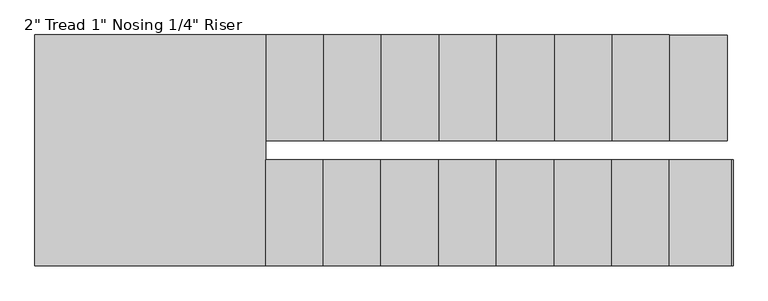
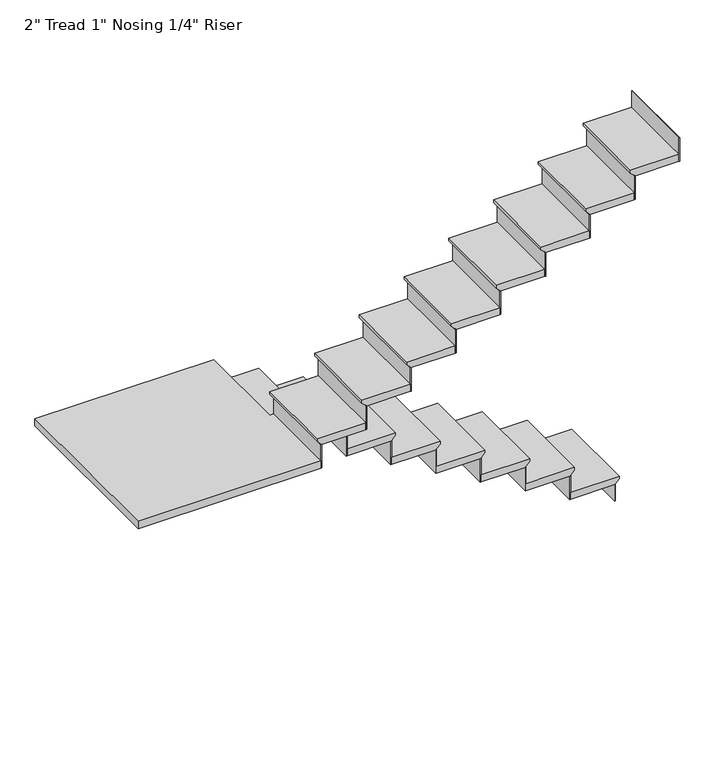
"""IFC4 building model written with IfcOpenShell, lengths in millimetres: stair flight geometry."""

from ifc_helpers import new_model, si_unit, origin, place, context, project, spatial, faceted_brep, source, transform, mapped, element, save


def stair_flight_bb5844b6(model_context):
    return source(origin(), model_context, "Body", "Brep", [
        faceted_brep([(-1805.9198569, -5306.3933037, 150.2833333), (-1805.9198569, -5306.3933037, 169.3333333), (-1805.9198569, -5865.1933037, 169.3333333), (-1805.9198569, -5865.1933037, 150.2833333), (-1831.3198569, -5306.3933037, 124.8833333), (-1831.3198569, -5865.1933037, 124.8833333), (-2136.1198569, -5306.3933037, 169.3333333), (-2136.1198569, -5865.1933037, 169.3333333), (-1831.3198569, -5865.1933037, 118.5333333), (-2136.1198569, -5865.1933037, 118.5333333), (-2136.1198569, -5306.3933037, 118.5333333), (-1831.3198569, -5306.3933037, 118.5333333)], [[[0, 1, 2, 3]], [[4, 0, 3, 5]], [[2, 1, 6, 7]], [[8, 9, 10, 11]], [[2, 7, 9, 8, 5, 3]], [[8, 11, 4, 5]], [[6, 1, 0, 4, 11, 10]], [[7, 6, 10, 9]]]),
        faceted_brep([(-1831.3198569, -5306.3933037, 118.5333333), (-1831.3198569, -5306.3933037, 0.0), (-1837.6698569, -5306.3933037, 0.0), (-1837.6698569, -5306.3933037, 118.5333333), (-1831.3198569, -5865.1933037, 118.5333333), (-1837.6698569, -5865.1933037, 118.5333333), (-1837.6698569, -5865.1933037, 0.0), (-1831.3198569, -5865.1933037, 0.0)], [[[0, 1, 2, 3]], [[4, 5, 6, 7]], [[1, 0, 4, 7]], [[2, 1, 7, 6]], [[3, 2, 6, 5]], [[0, 3, 5, 4]]]),
        faceted_brep([(-2136.1198569, -5306.3933037, 287.8666667), (-2136.1198569, -5306.3933037, 118.5333333), (-2142.4698569, -5306.3933037, 118.5333333), (-2142.4698569, -5306.3933037, 287.8666667), (-2136.1198569, -5865.1933037, 287.8666667), (-2142.4698569, -5865.1933037, 287.8666667), (-2142.4698569, -5865.1933037, 118.5333333), (-2136.1198569, -5865.1933037, 118.5333333)], [[[0, 1, 2, 3]], [[4, 5, 6, 7]], [[1, 0, 4, 7]], [[2, 1, 7, 6]], [[3, 2, 6, 5]], [[0, 3, 5, 4]]]),
        faceted_brep([(-2110.7198569, -5865.1933037, 338.6666667), (-2110.7198569, -5306.3933037, 338.6666667), (-2440.9198569, -5306.3933037, 338.6666667), (-2440.9198569, -5865.1933037, 338.6666667), (-2136.1198569, -5865.1933037, 287.8666667), (-2440.9198569, -5865.1933037, 287.8666667), (-2440.9198569, -5306.3933037, 287.8666667), (-2136.1198569, -5306.3933037, 287.8666667), (-2136.1198569, -5865.1933037, 294.2166667), (-2110.7198569, -5865.1933037, 319.6166667), (-2136.1198569, -5306.3933037, 294.2166667), (-2110.7198569, -5306.3933037, 319.6166667)], [[[0, 1, 2, 3]], [[4, 5, 6, 7]], [[0, 3, 5, 4, 8, 9]], [[4, 7, 10, 8]], [[2, 1, 11, 10, 7, 6]], [[3, 2, 6, 5]], [[11, 1, 0, 9]], [[10, 11, 9, 8]]]),
        faceted_brep([(-2440.9198569, -5306.3933037, 457.2), (-2440.9198569, -5306.3933037, 287.8666667), (-2447.2698569, -5306.3933037, 287.8666667), (-2447.2698569, -5306.3933037, 457.2), (-2440.9198569, -5865.1933037, 457.2), (-2447.2698569, -5865.1933037, 457.2), (-2447.2698569, -5865.1933037, 287.8666667), (-2440.9198569, -5865.1933037, 287.8666667)], [[[0, 1, 2, 3]], [[4, 5, 6, 7]], [[1, 0, 4, 7]], [[2, 1, 7, 6]], [[3, 2, 6, 5]], [[0, 3, 5, 4]]]),
        faceted_brep([(-2415.5198569, -5865.1933037, 508.0), (-2415.5198569, -5306.3933037, 508.0), (-2745.7198569, -5306.3933037, 508.0), (-2745.7198569, -5865.1933037, 508.0), (-2440.9198569, -5865.1933037, 457.2), (-2745.7198569, -5865.1933037, 457.2), (-2745.7198569, -5306.3933037, 457.2), (-2440.9198569, -5306.3933037, 457.2), (-2440.9198569, -5865.1933037, 463.55), (-2415.5198569, -5865.1933037, 488.95), (-2440.9198569, -5306.3933037, 463.55), (-2415.5198569, -5306.3933037, 488.95)], [[[0, 1, 2, 3]], [[4, 5, 6, 7]], [[0, 3, 5, 4, 8, 9]], [[4, 7, 10, 8]], [[2, 1, 11, 10, 7, 6]], [[3, 2, 6, 5]], [[11, 1, 0, 9]], [[10, 11, 9, 8]]]),
        faceted_brep([(-2745.7198569, -5306.3933037, 626.5333333), (-2745.7198569, -5306.3933037, 457.2), (-2752.0698569, -5306.3933037, 457.2), (-2752.0698569, -5306.3933037, 626.5333333), (-2745.7198569, -5865.1933037, 626.5333333), (-2752.0698569, -5865.1933037, 626.5333333), (-2752.0698569, -5865.1933037, 457.2), (-2745.7198569, -5865.1933037, 457.2)], [[[0, 1, 2, 3]], [[4, 5, 6, 7]], [[1, 0, 4, 7]], [[2, 1, 7, 6]], [[3, 2, 6, 5]], [[0, 3, 5, 4]]]),
        faceted_brep([(-2720.3198569, -5865.1933037, 677.3333333), (-2720.3198569, -5306.3933037, 677.3333333), (-3050.5198569, -5306.3933037, 677.3333333), (-3050.5198569, -5865.1933037, 677.3333333), (-2745.7198569, -5865.1933037, 626.5333333), (-3050.5198569, -5865.1933037, 626.5333333), (-3050.5198569, -5306.3933037, 626.5333333), (-2745.7198569, -5306.3933037, 626.5333333), (-2745.7198569, -5865.1933037, 632.8833333), (-2720.3198569, -5865.1933037, 658.2833333), (-2745.7198569, -5306.3933037, 632.8833333), (-2720.3198569, -5306.3933037, 658.2833333)], [[[0, 1, 2, 3]], [[4, 5, 6, 7]], [[0, 3, 5, 4, 8, 9]], [[4, 7, 10, 8]], [[2, 1, 11, 10, 7, 6]], [[3, 2, 6, 5]], [[11, 1, 0, 9]], [[10, 11, 9, 8]]]),
        faceted_brep([(-3050.5198569, -5306.3933037, 795.8666667), (-3050.5198569, -5306.3933037, 626.5333333), (-3056.8698569, -5306.3933037, 626.5333333), (-3056.8698569, -5306.3933037, 795.8666667), (-3050.5198569, -5865.1933037, 795.8666667), (-3056.8698569, -5865.1933037, 795.8666667), (-3056.8698569, -5865.1933037, 626.5333333), (-3050.5198569, -5865.1933037, 626.5333333)], [[[0, 1, 2, 3]], [[4, 5, 6, 7]], [[1, 0, 4, 7]], [[2, 1, 7, 6]], [[3, 2, 6, 5]], [[0, 3, 5, 4]]]),
        faceted_brep([(-3025.1198569, -5865.1933037, 846.6666667), (-3025.1198569, -5306.3933037, 846.6666667), (-3355.3198569, -5306.3933037, 846.6666667), (-3355.3198569, -5865.1933037, 846.6666667), (-3050.5198569, -5865.1933037, 795.8666667), (-3355.3198569, -5865.1933037, 795.8666667), (-3355.3198569, -5306.3933037, 795.8666667), (-3050.5198569, -5306.3933037, 795.8666667), (-3050.5198569, -5865.1933037, 802.2166667), (-3025.1198569, -5865.1933037, 827.6166667), (-3050.5198569, -5306.3933037, 802.2166667), (-3025.1198569, -5306.3933037, 827.6166667)], [[[0, 1, 2, 3]], [[4, 5, 6, 7]], [[0, 3, 5, 4, 8, 9]], [[4, 7, 10, 8]], [[2, 1, 11, 10, 7, 6]], [[3, 2, 6, 5]], [[11, 1, 0, 9]], [[10, 11, 9, 8]]]),
        faceted_brep([(-3355.3198569, -5306.3933037, 965.2), (-3355.3198569, -5306.3933037, 795.8666667), (-3361.6698569, -5306.3933037, 795.8666667), (-3361.6698569, -5306.3933037, 965.2), (-3355.3198569, -5865.1933037, 965.2), (-3361.6698569, -5865.1933037, 965.2), (-3361.6698569, -5865.1933037, 795.8666667), (-3355.3198569, -5865.1933037, 795.8666667)], [[[0, 1, 2, 3]], [[4, 5, 6, 7]], [[1, 0, 4, 7]], [[2, 1, 7, 6]], [[3, 2, 6, 5]], [[0, 3, 5, 4]]]),
        faceted_brep([(-3329.9198569, -5865.1933037, 1016.0), (-3329.9198569, -5306.3933037, 1016.0), (-3660.1198569, -5306.3933037, 1016.0), (-3660.1198569, -5865.1933037, 1016.0), (-3355.3198569, -5865.1933037, 965.2), (-3660.1198569, -5865.1933037, 965.2), (-3660.1198569, -5306.3933037, 965.2), (-3355.3198569, -5306.3933037, 965.2), (-3355.3198569, -5865.1933037, 971.55), (-3329.9198569, -5865.1933037, 996.95), (-3355.3198569, -5306.3933037, 971.55), (-3329.9198569, -5306.3933037, 996.95)], [[[0, 1, 2, 3]], [[4, 5, 6, 7]], [[0, 3, 5, 4, 8, 9]], [[4, 7, 10, 8]], [[2, 1, 11, 10, 7, 6]], [[3, 2, 6, 5]], [[11, 1, 0, 9]], [[10, 11, 9, 8]]]),
        faceted_brep([(-3660.1198569, -5306.3933037, 1134.5333333), (-3660.1198569, -5306.3933037, 965.2), (-3666.4698569, -5306.3933037, 965.2), (-3666.4698569, -5306.3933037, 1134.5333333), (-3660.1198569, -5865.1933037, 1134.5333333), (-3666.4698569, -5865.1933037, 1134.5333333), (-3666.4698569, -5865.1933037, 965.2), (-3660.1198569, -5865.1933037, 965.2)], [[[0, 1, 2, 3]], [[4, 5, 6, 7]], [[1, 0, 4, 7]], [[2, 1, 7, 6]], [[3, 2, 6, 5]], [[0, 3, 5, 4]]]),
        faceted_brep([(-3634.7198569, -5865.1933037, 1185.3333333), (-3634.7198569, -5306.3933037, 1185.3333333), (-3964.9198569, -5306.3933037, 1185.3333333), (-3964.9198569, -5865.1933037, 1185.3333333), (-3660.1198569, -5865.1933037, 1134.5333333), (-3964.9198569, -5865.1933037, 1134.5333333), (-3964.9198569, -5306.3933037, 1134.5333333), (-3660.1198569, -5306.3933037, 1134.5333333), (-3660.1198569, -5865.1933037, 1140.8833333), (-3634.7198569, -5865.1933037, 1166.2833333), (-3660.1198569, -5306.3933037, 1140.8833333), (-3634.7198569, -5306.3933037, 1166.2833333)], [[[0, 1, 2, 3]], [[4, 5, 6, 7]], [[0, 3, 5, 4, 8, 9]], [[4, 7, 10, 8]], [[2, 1, 11, 10, 7, 6]], [[3, 2, 6, 5]], [[11, 1, 0, 9]], [[10, 11, 9, 8]]]),
        faceted_brep([(-3964.9198569, -5306.3933037, 1303.8666667), (-3964.9198569, -5306.3933037, 1134.5333333), (-3971.2698569, -5306.3933037, 1134.5333333), (-3971.2698569, -5306.3933037, 1303.8666667), (-3964.9198569, -5865.1933037, 1303.8666667), (-3971.2698569, -5865.1933037, 1303.8666667), (-3971.2698569, -5865.1933037, 1134.5333333), (-3964.9198569, -5865.1933037, 1134.5333333)], [[[0, 1, 2, 3]], [[4, 5, 6, 7]], [[1, 0, 4, 7]], [[2, 1, 7, 6]], [[3, 2, 6, 5]], [[0, 3, 5, 4]]]),
        faceted_brep([(-3939.5198569, -5865.1933037, 1354.6666667), (-3939.5198569, -5306.3933037, 1354.6666667), (-4269.7198569, -5306.3933037, 1354.6666667), (-4269.7198569, -5865.1933037, 1354.6666667), (-3964.9198569, -5865.1933037, 1303.8666667), (-4269.7198569, -5865.1933037, 1303.8666667), (-4269.7198569, -5306.3933037, 1303.8666667), (-3964.9198569, -5306.3933037, 1303.8666667), (-3964.9198569, -5865.1933037, 1310.2166667), (-3939.5198569, -5865.1933037, 1335.6166667), (-3964.9198569, -5306.3933037, 1310.2166667), (-3939.5198569, -5306.3933037, 1335.6166667)], [[[0, 1, 2, 3]], [[4, 5, 6, 7]], [[0, 3, 5, 4, 8, 9]], [[4, 7, 10, 8]], [[2, 1, 11, 10, 7, 6]], [[3, 2, 6, 5]], [[11, 1, 0, 9]], [[10, 11, 9, 8]]]),
        faceted_brep([(-4269.7198569, -5306.3933037, 1473.2), (-4269.7198569, -5306.3933037, 1303.8666667), (-4276.0698569, -5306.3933037, 1303.8666667), (-4276.0698569, -5306.3933037, 1473.2), (-4269.7198569, -5865.1933037, 1473.2), (-4276.0698569, -5865.1933037, 1473.2), (-4276.0698569, -5865.1933037, 1303.8666667), (-4269.7198569, -5865.1933037, 1303.8666667)], [[[0, 1, 2, 3]], [[4, 5, 6, 7]], [[1, 0, 4, 7]], [[2, 1, 7, 6]], [[3, 2, 6, 5]], [[0, 3, 5, 4]]]),
        faceted_brep([(-4218.9198569, -5966.7933037, 1524.0), (-4244.3198569, -5966.7933037, 1524.0), (-4244.3198569, -5306.3933037, 1524.0), (-5463.5198569, -5306.3933037, 1524.0), (-5463.5198569, -6525.5933037, 1524.0), (-4218.9198569, -6525.5933037, 1524.0), (-4244.3198569, -5966.7933037, 1473.2), (-4218.9198569, -5966.7933037, 1473.2), (-4218.9198569, -6525.5933037, 1473.2), (-5463.5198569, -6525.5933037, 1473.2), (-5463.5198569, -5306.3933037, 1473.2), (-4269.7198569, -5306.3933037, 1473.2), (-4269.7198569, -5865.1933037, 1473.2), (-4244.3198569, -5865.1933037, 1473.2), (-4244.3198569, -5865.1933037, 1504.95), (-4244.3198569, -5306.3933037, 1504.95), (-4269.7198569, -5865.1933037, 1479.55), (-4269.7198569, -5306.3933037, 1479.55)], [[[0, 1, 2, 3, 4, 5]], [[6, 7, 8, 9, 10, 11, 12, 13]], [[1, 0, 7, 6]], [[2, 1, 6, 13, 14, 15]], [[13, 12, 16, 14]], [[12, 11, 17, 16]], [[3, 2, 15, 17, 11, 10]], [[4, 3, 10, 9]], [[5, 4, 9, 8]], [[0, 5, 8, 7]], [[17, 15, 14, 16]]]),
        faceted_brep([(-4218.9198569, -6525.5933037, 1642.5333333), (-4218.9198569, -6525.5933037, 1473.2), (-4212.5698569, -6525.5933037, 1473.2), (-4212.5698569, -6525.5933037, 1642.5333333), (-4218.9198569, -5966.7933037, 1642.5333333), (-4212.5698569, -5966.7933037, 1642.5333333), (-4212.5698569, -5966.7933037, 1473.2), (-4218.9198569, -5966.7933037, 1473.2)], [[[0, 1, 2, 3]], [[4, 5, 6, 7]], [[1, 0, 4, 7]], [[2, 1, 7, 6]], [[3, 2, 6, 5]], [[0, 3, 5, 4]]]),
        faceted_brep([(-4244.3198569, -5966.7933037, 1693.3333333), (-4244.3198569, -6525.5933037, 1693.3333333), (-3914.1198569, -6525.5933037, 1693.3333333), (-3914.1198569, -5966.7933037, 1693.3333333), (-4218.9198569, -5966.7933037, 1642.5333333), (-3914.1198569, -5966.7933037, 1642.5333333), (-3914.1198569, -6525.5933037, 1642.5333333), (-4218.9198569, -6525.5933037, 1642.5333333), (-4218.9198569, -5966.7933037, 1648.8833333), (-4244.3198569, -5966.7933037, 1674.2833333), (-4218.9198569, -6525.5933037, 1648.8833333), (-4244.3198569, -6525.5933037, 1674.2833333)], [[[0, 1, 2, 3]], [[4, 5, 6, 7]], [[0, 3, 5, 4, 8, 9]], [[4, 7, 10, 8]], [[2, 1, 11, 10, 7, 6]], [[3, 2, 6, 5]], [[11, 1, 0, 9]], [[10, 11, 9, 8]]]),
        faceted_brep([(-3914.1198569, -6525.5933037, 1811.8666667), (-3914.1198569, -6525.5933037, 1642.5333333), (-3907.7698569, -6525.5933037, 1642.5333333), (-3907.7698569, -6525.5933037, 1811.8666667), (-3914.1198569, -5966.7933037, 1811.8666667), (-3907.7698569, -5966.7933037, 1811.8666667), (-3907.7698569, -5966.7933037, 1642.5333333), (-3914.1198569, -5966.7933037, 1642.5333333)], [[[0, 1, 2, 3]], [[4, 5, 6, 7]], [[1, 0, 4, 7]], [[2, 1, 7, 6]], [[3, 2, 6, 5]], [[0, 3, 5, 4]]]),
        faceted_brep([(-3939.5198569, -5966.7933037, 1862.6666667), (-3939.5198569, -6525.5933037, 1862.6666667), (-3609.3198569, -6525.5933037, 1862.6666667), (-3609.3198569, -5966.7933037, 1862.6666667), (-3914.1198569, -5966.7933037, 1811.8666667), (-3609.3198569, -5966.7933037, 1811.8666667), (-3609.3198569, -6525.5933037, 1811.8666667), (-3914.1198569, -6525.5933037, 1811.8666667), (-3914.1198569, -5966.7933037, 1818.2166667), (-3939.5198569, -5966.7933037, 1843.6166667), (-3914.1198569, -6525.5933037, 1818.2166667), (-3939.5198569, -6525.5933037, 1843.6166667)], [[[0, 1, 2, 3]], [[4, 5, 6, 7]], [[0, 3, 5, 4, 8, 9]], [[4, 7, 10, 8]], [[2, 1, 11, 10, 7, 6]], [[3, 2, 6, 5]], [[11, 1, 0, 9]], [[10, 11, 9, 8]]]),
        faceted_brep([(-3609.3198569, -6525.5933037, 1981.2), (-3609.3198569, -6525.5933037, 1811.8666667), (-3602.9698569, -6525.5933037, 1811.8666667), (-3602.9698569, -6525.5933037, 1981.2), (-3609.3198569, -5966.7933037, 1981.2), (-3602.9698569, -5966.7933037, 1981.2), (-3602.9698569, -5966.7933037, 1811.8666667), (-3609.3198569, -5966.7933037, 1811.8666667)], [[[0, 1, 2, 3]], [[4, 5, 6, 7]], [[1, 0, 4, 7]], [[2, 1, 7, 6]], [[3, 2, 6, 5]], [[0, 3, 5, 4]]]),
        faceted_brep([(-3634.7198569, -5966.7933037, 2032.0), (-3634.7198569, -6525.5933037, 2032.0), (-3304.5198569, -6525.5933037, 2032.0), (-3304.5198569, -5966.7933037, 2032.0), (-3609.3198569, -5966.7933037, 1981.2), (-3304.5198569, -5966.7933037, 1981.2), (-3304.5198569, -6525.5933037, 1981.2), (-3609.3198569, -6525.5933037, 1981.2), (-3609.3198569, -5966.7933037, 1987.55), (-3634.7198569, -5966.7933037, 2012.95), (-3609.3198569, -6525.5933037, 1987.55), (-3634.7198569, -6525.5933037, 2012.95)], [[[0, 1, 2, 3]], [[4, 5, 6, 7]], [[0, 3, 5, 4, 8, 9]], [[4, 7, 10, 8]], [[2, 1, 11, 10, 7, 6]], [[3, 2, 6, 5]], [[11, 1, 0, 9]], [[10, 11, 9, 8]]]),
        faceted_brep([(-3304.5198569, -6525.5933037, 2150.5333333), (-3304.5198569, -6525.5933037, 1981.2), (-3298.1698569, -6525.5933037, 1981.2), (-3298.1698569, -6525.5933037, 2150.5333333), (-3304.5198569, -5966.7933037, 2150.5333333), (-3298.1698569, -5966.7933037, 2150.5333333), (-3298.1698569, -5966.7933037, 1981.2), (-3304.5198569, -5966.7933037, 1981.2)], [[[0, 1, 2, 3]], [[4, 5, 6, 7]], [[1, 0, 4, 7]], [[2, 1, 7, 6]], [[3, 2, 6, 5]], [[0, 3, 5, 4]]]),
        faceted_brep([(-3329.9198569, -5966.7933037, 2201.3333333), (-3329.9198569, -6525.5933037, 2201.3333333), (-2999.7198569, -6525.5933037, 2201.3333333), (-2999.7198569, -5966.7933037, 2201.3333333), (-3304.5198569, -5966.7933037, 2150.5333333), (-2999.7198569, -5966.7933037, 2150.5333333), (-2999.7198569, -6525.5933037, 2150.5333333), (-3304.5198569, -6525.5933037, 2150.5333333), (-3304.5198569, -5966.7933037, 2156.8833333), (-3329.9198569, -5966.7933037, 2182.2833333), (-3304.5198569, -6525.5933037, 2156.8833333), (-3329.9198569, -6525.5933037, 2182.2833333)], [[[0, 1, 2, 3]], [[4, 5, 6, 7]], [[0, 3, 5, 4, 8, 9]], [[4, 7, 10, 8]], [[2, 1, 11, 10, 7, 6]], [[3, 2, 6, 5]], [[11, 1, 0, 9]], [[10, 11, 9, 8]]]),
        faceted_brep([(-2999.7198569, -6525.5933037, 2319.8666667), (-2999.7198569, -6525.5933037, 2150.5333333), (-2993.3698569, -6525.5933037, 2150.5333333), (-2993.3698569, -6525.5933037, 2319.8666667), (-2999.7198569, -5966.7933037, 2319.8666667), (-2993.3698569, -5966.7933037, 2319.8666667), (-2993.3698569, -5966.7933037, 2150.5333333), (-2999.7198569, -5966.7933037, 2150.5333333)], [[[0, 1, 2, 3]], [[4, 5, 6, 7]], [[1, 0, 4, 7]], [[2, 1, 7, 6]], [[3, 2, 6, 5]], [[0, 3, 5, 4]]]),
        faceted_brep([(-3025.1198569, -5966.7933037, 2370.6666667), (-3025.1198569, -6525.5933037, 2370.6666667), (-2694.9198569, -6525.5933037, 2370.6666667), (-2694.9198569, -5966.7933037, 2370.6666667), (-2999.7198569, -5966.7933037, 2319.8666667), (-2694.9198569, -5966.7933037, 2319.8666667), (-2694.9198569, -6525.5933037, 2319.8666667), (-2999.7198569, -6525.5933037, 2319.8666667), (-2999.7198569, -5966.7933037, 2326.2166667), (-3025.1198569, -5966.7933037, 2351.6166667), (-2999.7198569, -6525.5933037, 2326.2166667), (-3025.1198569, -6525.5933037, 2351.6166667)], [[[0, 1, 2, 3]], [[4, 5, 6, 7]], [[0, 3, 5, 4, 8, 9]], [[4, 7, 10, 8]], [[2, 1, 11, 10, 7, 6]], [[3, 2, 6, 5]], [[11, 1, 0, 9]], [[10, 11, 9, 8]]]),
        faceted_brep([(-2694.9198569, -6525.5933037, 2489.2), (-2694.9198569, -6525.5933037, 2319.8666667), (-2688.5698569, -6525.5933037, 2319.8666667), (-2688.5698569, -6525.5933037, 2489.2), (-2694.9198569, -5966.7933037, 2489.2), (-2688.5698569, -5966.7933037, 2489.2), (-2688.5698569, -5966.7933037, 2319.8666667), (-2694.9198569, -5966.7933037, 2319.8666667)], [[[0, 1, 2, 3]], [[4, 5, 6, 7]], [[1, 0, 4, 7]], [[2, 1, 7, 6]], [[3, 2, 6, 5]], [[0, 3, 5, 4]]]),
        faceted_brep([(-2720.3198569, -5966.7933037, 2540.0), (-2720.3198569, -6525.5933037, 2540.0), (-2390.1198569, -6525.5933037, 2540.0), (-2390.1198569, -5966.7933037, 2540.0), (-2694.9198569, -5966.7933037, 2489.2), (-2390.1198569, -5966.7933037, 2489.2), (-2390.1198569, -6525.5933037, 2489.2), (-2694.9198569, -6525.5933037, 2489.2), (-2694.9198569, -5966.7933037, 2495.55), (-2720.3198569, -5966.7933037, 2520.95), (-2694.9198569, -6525.5933037, 2495.55), (-2720.3198569, -6525.5933037, 2520.95)], [[[0, 1, 2, 3]], [[4, 5, 6, 7]], [[0, 3, 5, 4, 8, 9]], [[4, 7, 10, 8]], [[2, 1, 11, 10, 7, 6]], [[3, 2, 6, 5]], [[11, 1, 0, 9]], [[10, 11, 9, 8]]]),
        faceted_brep([(-2390.1198569, -6525.5933037, 2658.5333333), (-2390.1198569, -6525.5933037, 2489.2), (-2383.7698569, -6525.5933037, 2489.2), (-2383.7698569, -6525.5933037, 2658.5333333), (-2390.1198569, -5966.7933037, 2658.5333333), (-2383.7698569, -5966.7933037, 2658.5333333), (-2383.7698569, -5966.7933037, 2489.2), (-2390.1198569, -5966.7933037, 2489.2)], [[[0, 1, 2, 3]], [[4, 5, 6, 7]], [[1, 0, 4, 7]], [[2, 1, 7, 6]], [[3, 2, 6, 5]], [[0, 3, 5, 4]]]),
        faceted_brep([(-2415.5198569, -5966.7933037, 2709.3333333), (-2415.5198569, -6525.5933037, 2709.3333333), (-2085.3198569, -6525.5933037, 2709.3333333), (-2085.3198569, -5966.7933037, 2709.3333333), (-2390.1198569, -5966.7933037, 2658.5333333), (-2085.3198569, -5966.7933037, 2658.5333333), (-2085.3198569, -6525.5933037, 2658.5333333), (-2390.1198569, -6525.5933037, 2658.5333333), (-2390.1198569, -5966.7933037, 2664.8833333), (-2415.5198569, -5966.7933037, 2690.2833333), (-2390.1198569, -6525.5933037, 2664.8833333), (-2415.5198569, -6525.5933037, 2690.2833333)], [[[0, 1, 2, 3]], [[4, 5, 6, 7]], [[0, 3, 5, 4, 8, 9]], [[4, 7, 10, 8]], [[2, 1, 11, 10, 7, 6]], [[3, 2, 6, 5]], [[11, 1, 0, 9]], [[10, 11, 9, 8]]]),
        faceted_brep([(-2085.3198569, -6525.5933037, 2827.8666667), (-2085.3198569, -6525.5933037, 2658.5333333), (-2078.9698569, -6525.5933037, 2658.5333333), (-2078.9698569, -6525.5933037, 2827.8666667), (-2085.3198569, -5966.7933037, 2827.8666667), (-2078.9698569, -5966.7933037, 2827.8666667), (-2078.9698569, -5966.7933037, 2658.5333333), (-2085.3198569, -5966.7933037, 2658.5333333)], [[[0, 1, 2, 3]], [[4, 5, 6, 7]], [[1, 0, 4, 7]], [[2, 1, 7, 6]], [[3, 2, 6, 5]], [[0, 3, 5, 4]]]),
        faceted_brep([(-1780.5198569, -6525.5933037, 2997.2), (-1780.5198569, -6525.5933037, 2827.8666667), (-1774.1698569, -6525.5933037, 2827.8666667), (-1774.1698569, -6525.5933037, 2997.2), (-1780.5198569, -5966.7933037, 2997.2), (-1774.1698569, -5966.7933037, 2997.2), (-1774.1698569, -5966.7933037, 2827.8666667), (-1780.5198569, -5966.7933037, 2827.8666667)], [[[0, 1, 2, 3]], [[4, 5, 6, 7]], [[1, 0, 4, 7]], [[2, 1, 7, 6]], [[3, 2, 6, 5]], [[0, 3, 5, 4]]]),
        faceted_brep([(-2110.7198569, -5966.7933037, 2878.6666667), (-2110.7198569, -6525.5933037, 2878.6666667), (-1780.5198569, -6525.5933037, 2878.6666667), (-1780.5198569, -5966.7933037, 2878.6666667), (-2085.3198569, -5966.7933037, 2827.8666667), (-1780.5198569, -5966.7933037, 2827.8666667), (-1780.5198569, -6525.5933037, 2827.8666667), (-2085.3198569, -6525.5933037, 2827.8666667), (-2085.3198569, -5966.7933037, 2834.2166667), (-2110.7198569, -5966.7933037, 2859.6166667), (-2085.3198569, -6525.5933037, 2834.2166667), (-2110.7198569, -6525.5933037, 2859.6166667)], [[[0, 1, 2, 3]], [[4, 5, 6, 7]], [[0, 3, 5, 4, 8, 9]], [[4, 7, 10, 8]], [[2, 1, 11, 10, 7, 6]], [[3, 2, 6, 5]], [[11, 1, 0, 9]], [[10, 11, 9, 8]]]),
    ])


if __name__ == "__main__":
    model = new_model("IFC4")
    model_context = context("Model", 3, world=origin())
    ifc_project = project(units=[si_unit("LENGTHUNIT", "METRE", prefix="MILLI")], contexts=[model_context])
    site = spatial("IfcSite", under=ifc_project)
    building = spatial("IfcBuilding", under=site)
    placement = place(None, origin())
    stair_flight_shape = stair_flight_bb5844b6(model_context)
    element("IfcStairFlight", 1, ObjectType="2\" Tread 1\" Nosing 1/4\" Riser", at=placement, inside=building, context=model_context, shape_type="MappedRepresentation", body=[
        mapped(stair_flight_shape, transform((0.0, 0.0, 0.0), x_axis=(1.0, 0.0, 0.0), y_axis=(0.0, 1.0, 0.0), z_axis=(0.0, 0.0, 1.0))),
    ])
    save(model, "model.ifc")
